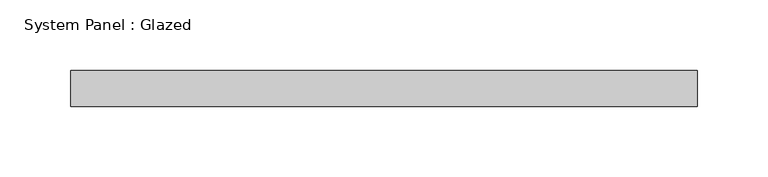
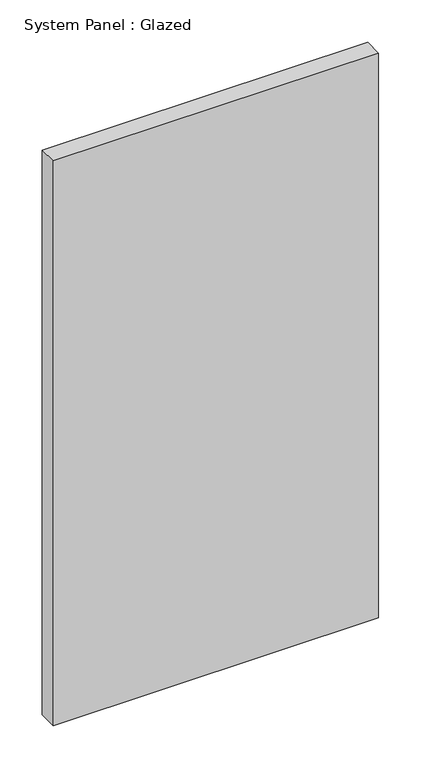
"""IFC4 building model written with IfcOpenShell, lengths in millimetres: plate geometry, System Panel : Glazed."""

from ifc_helpers import new_model, si_unit, origin, origin_with_axes, place, context, project, spatial, polyline, outline, extrude, source, transform, mapped, element, save


def system_panel_glazed_6562854e(model_context):
    return source(origin(), model_context, "Body", "SweptSolid", [
        extrude(outline(polyline([(221.7349132, 19.05), (-221.7349132, 19.05), (-221.7349132, 44.45), (221.7349132, 44.45), (221.7349132, 19.05)])), origin_with_axes(), (0.0, 0.0, 1.0), 812.8),
    ])


if __name__ == "__main__":
    model = new_model("IFC4")
    model_context = context("Model", 3, world=origin())
    ifc_project = project(units=[si_unit("LENGTHUNIT", "METRE", prefix="MILLI")], contexts=[model_context])
    site = spatial("IfcSite", under=ifc_project)
    building = spatial("IfcBuilding", under=site)
    placement = place(None, origin())
    system_panel_glazed_shape = system_panel_glazed_6562854e(model_context)
    element("IfcPlate", 1, ObjectType="System Panel : Glazed", at=placement, inside=building, context=model_context, shape_type="MappedRepresentation", body=[
        mapped(system_panel_glazed_shape, transform((0.0, 0.0, 0.0), x_axis=(1.0, 0.0, 0.0), y_axis=(0.0, 1.0, 0.0), z_axis=(0.0, 0.0, 1.0))),
    ])
    save(model, "model.ifc")

# Revit data of these elements
# Type "System Panel : Glazed"
#   Construction Type Id = "GSP4R"
#   Analytic Construction = "1/8 in Pilkington single glazing"
#   Visual Light Transmittance = 0.9
#   Solar Heat Gain Coefficient = 0.86
#   Heat Transfer Coefficient (U) = 1.18115 BTU/(h·ft²·°F)
# Element 1 (IfcPlate, "System Panel : Glazed")
#   Materials on its faces: "Glass"
# Materials
#   "Glass": class "Glass", colour RGB 0 128 192, transparency 0.75, Description = "Soda Lime Glass", Cost = 0
